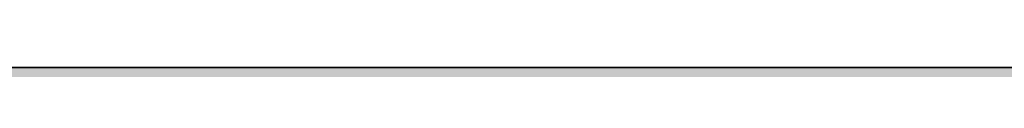
# Model space of a CAD drawing. Units: inches. Extents: x 2091 to 2899, y 967 to 2217.
# Tile 89 of 256: x 2251.29649 to 2251.31428, y 1099.91903 to 1099.91922. Entities that reach past the tile are written whole.
import ezdxf

# ---------------------------------------------------------------- set-up
doc = ezdxf.new("R2010")
doc.units = ezdxf.units.IN
doc.layers.add('A-WALL-PATT', color=141, linetype='Continuous', lineweight=13, true_color=0xadddf7)
doc.layers.add('L-SITE-WALL', color=7, linetype='Continuous', lineweight=35)

msp = doc.modelspace()

# ---------------------------------------------------------------- hatches: boundary and pattern name
at = {"layer": 'A-WALL-PATT'}
h = msp.add_hatch(color=256, dxfattribs=at)
h.dxf.hatch_style = 1
h.paths.add_polyline_path([(2212.143603, 1941.419059), (2387.643603, 1941.419059), (2387.643603, 1824.419059), (2392.143603, 1824.419059), (2392.143603, 1941.419059), (2609.643603, 1941.419059), (2609.643603, 1825.919059), (2614.143603, 1825.919059), (2614.143603, 1941.419059), (2794.143603, 1941.419059), (2794.143603, 1928.762166), (2803.143603, 1928.762166), (2803.143603, 2050.919059), (2203.143603, 2050.919059), (2203.143603, 1900.757859), (2212.143603, 1900.757859)])
h.paths.add_polyline_path([(2212.143603, 1945.919059), (2212.143603, 2041.919059), (2794.143603, 2041.919059), (2794.143603, 1945.919059), (2402.248245, 1945.919059), (2401.102434, 1945.775832), (2398.702434, 1945.775832)], flags=16)
h.paths.add_polyline_path([(2230.229861, 1948.062793), (2227.349861, 1949.502793), (2225.909861, 1951.902793), (2223.989861, 1952.862793), (2223.029861, 1955.262793), (2222.069861, 1959.582793), (2222.069861, 1963.422793), (2223.029861, 1965.662793), (2223.989861, 1965.342793), (2225.58591, 1963.860747), (2226.911533, 1964.957259), (2226.948861, 1965.938793), (2227.778319, 1966.952143), (2228.199916, 1968.878704), (2230.709861, 1964.862793), (2233.589861, 1966.302793), (2233.607309, 1966.331873), (2233.772659, 1964.938205), (2234.633802, 1963.676473), (2235.029861, 1963.902793), (2236.282035, 1965.572358), (2235.989861, 1962.942793), (2237.954512, 1957.540002), (2238.389861, 1957.902793), (2239.215861, 1960.305793), (2238.654565, 1966.38496), (2238.692792, 1966.438069), (2238.840578, 1967.499707), (2238.780291, 1967.687486), (2238.880538, 1967.786763), (2238.666861, 1966.251793), (2239.215861, 1960.305793), (2238.389861, 1957.902793), (2236.949861, 1956.702793), (2234.549861, 1949.982793)], flags=0)
h.paths.add_polyline_path([(2278.011974, 1948.062793), (2276.496427, 1947.873349), (2275.849833, 1947.688608), (2274.651974, 1947.102793)], flags=0)
h.paths.add_polyline_path([(2269.851974, 1955.742793), (2268.276176, 1956.629329), (2270.867302, 1956.348398), (2269.371974, 1958.142793), (2268.714964, 1959.192325), (2270.569833, 1958.728608), (2268.580725, 1961.906087), (2270.811974, 1960.891883), (2270.811974, 1963.422793), (2271.393315, 1964.779256), (2270.291762, 1966.156196), (2271.771974, 1965.662793), (2272.141387, 1966.524757), (2273.929833, 1965.928608), (2275.630385, 1968.054299), (2276.331938, 1966.72186), (2276.520431, 1966.952143), (2276.942029, 1968.878704), (2277.734293, 1967.611082), (2278.139888, 1969.46452), (2279.659124, 1967.033742), (2280.411974, 1966.782793), (2280.949302, 1967.588785), (2281.609833, 1967.368608), (2282.133266, 1968.153758), (2282.349235, 1966.333445), (2282.349849, 1966.332585), (2283.40755, 1968.09542), (2283.712631, 1965.52402), (2284.320221, 1964.633789), (2284.511809, 1964.889239), (2284.234974, 1965.704793), (2284.500472, 1967.318958), (2284.907944, 1965.41742), (2285.396313, 1966.068579), (2285.432833, 1966.290608), (2285.473338, 1966.171279), (2286.353919, 1967.345387), (2286.222007, 1966.158173), (2287.663492, 1968.080154), (2287.713974, 1968.442793), (2288.481599, 1969.016679), (2288.573993, 1968.728897), (2288.917461, 1969.06904), (2288.606833, 1966.837608), (2288.928726, 1963.35131), (2288.934974, 1963.356793), (2288.929731, 1963.340422), (2289.015281, 1962.413869), (2290.111223, 1963.875126), (2290.132833, 1963.942608), (2290.217672, 1964.017058), (2290.111223, 1963.875126), (2289.155833, 1960.891608), (2288.594036, 1959.257227), (2288.571974, 1959.102793), (2289.531974, 1960.542793), (2290.011974, 1962.462793), (2290.19184, 1962.642659), (2289.769833, 1959.688608), (2286.889833, 1957.288608), (2284.489833, 1950.568608), (2283.314658, 1950.046308), (2283.291974, 1949.982793), (2280.290059, 1948.648608), (2281.129833, 1948.648608), (2282.569833, 1948.168608), (2283.204726, 1948.062793), (2278.971974, 1948.062793), (2276.091974, 1949.502793), (2274.651974, 1951.902793), (2272.731974, 1952.862793)], flags=0)
h.paths.add_polyline_path([(2271.158868, 1958.021765), (2272.969833, 1955.848608), (2272.009833, 1960.168608), (2272.009833, 1964.008608), (2272.624426, 1965.442658), (2274.328023, 1963.860747), (2275.653646, 1964.957259), (2275.637743, 1964.53909), (2277.412231, 1966.006888), (2277.032974, 1965.156793), (2276.829924, 1964.975597), (2276.766012, 1963.295014), (2277.449635, 1962.66022), (2279.451974, 1964.862793), (2282.331974, 1966.302793), (2283.529833, 1966.888608), (2283.294512, 1966.770948), (2283.912993, 1963.8847), (2284.899249, 1964.448275), (2284.731974, 1962.942793), (2286.696625, 1957.540002), (2287.131974, 1957.902793), (2287.541913, 1959.095388), (2287.779395, 1958.442311), (2285.682738, 1956.695097), (2285.876503, 1959.795336), (2284.731974, 1962.942793), (2284.899249, 1964.448275), (2283.912993, 1963.8847), (2284.223833, 1962.434116), (2283.424365, 1963.605484), (2281.609833, 1962.568608), (2281.129833, 1960.168608), (2282.089833, 1956.328608), (2283.049833, 1952.968608), (2282.569833, 1950.568608), (2280.169833, 1948.648608), (2279.883316, 1948.791867), (2278.971974, 1948.062793), (2278.971974, 1949.022793), (2278.672313, 1949.397368), (2277.289833, 1950.088608), (2275.849833, 1952.488608), (2273.929833, 1953.448608), (2272.489833, 1954.888608), (2271.921647, 1954.888608), (2271.771974, 1955.262793)], flags=0)
h.paths.add_polyline_path([(2311.994146, 1955.742793), (2312.062717, 1955.674221), (2312.0551, 1955.7085)], flags=0)
h.paths.add_polyline_path([(2331.956146, 1963.951793), (2333.396146, 1965.391793), (2331.077146, 1963.356793), (2330.998603, 1963.111517)], flags=0)
h.paths.add_polyline_path([(2310.554146, 1954.302793), (2307.039807, 1956.279943), (2310.762903, 1955.876284), (2312.474146, 1953.822793), (2313.434146, 1951.422793), (2315.354146, 1950.462793), (2316.794146, 1948.062793), (2317.466146, 1947.726793), (2319.368691, 1947.964611), (2317.754146, 1949.982793), (2317.569531, 1950.610485), (2316.794146, 1951.902793), (2314.874146, 1952.862793), (2313.914146, 1955.262793), (2311.514146, 1958.142793), (2309.375489, 1961.559168), (2311.514146, 1960.337078), (2311.514146, 1961.982793), (2310.604672, 1963.119635), (2311.726605, 1962.47853), (2312.418332, 1964.09256), (2312.255964, 1964.29552), (2313.194146, 1963.982793), (2313.914146, 1965.662793), (2314.646778, 1965.418582), (2315.354146, 1966.302793), (2316.794146, 1967.742793), (2316.157435, 1966.946904), (2317.034111, 1965.28186), (2317.222604, 1965.512143), (2317.777048, 1968.045771), (2318.474111, 1966.72186), (2318.662604, 1966.952143), (2319.084201, 1968.878704), (2321.207049, 1965.482147), (2322.161419, 1966.913702), (2322.554146, 1966.782793), (2322.785988, 1967.130555), (2322.881646, 1966.324293), (2323.312041, 1965.72174), (2323.651289, 1965.891364), (2324.3965, 1967.133382), (2324.656945, 1964.938205), (2324.971986, 1964.476611), (2325.38728, 1967.001499), (2325.940813, 1964.418348), (2327.228929, 1966.135836), (2327.16632, 1965.572358), (2328.059139, 1966.762783), (2328.224576, 1966.247486), (2329.667971, 1967.67691), (2329.664576, 1967.687486), (2329.764823, 1967.786763), (2329.551146, 1966.251793), (2330.100146, 1960.305793), (2329.332814, 1958.07347), (2329.313065, 1957.935225), (2329.634146, 1958.202793), (2330.234146, 1959.102793), (2330.714146, 1961.022793), (2331.034146, 1961.342793), (2330.714146, 1959.102793), (2329.634146, 1958.202793), (2329.274146, 1957.662793), (2327.712112, 1956.361098), (2325.434146, 1949.982793), (2324.333769, 1949.493736), (2323.994146, 1948.542793), (2319.674146, 1946.622793), (2316.794146, 1948.062793), (2315.354146, 1950.462793), (2313.434146, 1951.422793)], flags=0)
h.paths.add_polyline_path([(2321.335684, 1947.952023), (2321.114146, 1948.062793), (2321.114146, 1949.022793), (2319.194146, 1951.422793), (2316.794146, 1959.582793), (2316.663237, 1959.582793), (2315.354146, 1958.142793), (2314.394146, 1958.142793), (2313.148303, 1958.709085), (2312.954146, 1959.582793), (2312.954146, 1960.891883), (2315.834146, 1959.582793), (2316.663237, 1959.582793), (2317.314709, 1960.299412), (2315.030195, 1962.420747), (2316.355818, 1963.517259), (2316.372337, 1963.951615), (2316.470195, 1963.860747), (2317.795818, 1964.957259), (2317.755219, 1963.889687), (2319.175146, 1965.156793), (2319.498407, 1965.881372), (2321.114146, 1965.342793), (2323.235885, 1962.372358), (2325.686349, 1963.772623), (2325.542789, 1962.480576), (2325.198783, 1963.494014), (2324.47851, 1963.082429), (2324.926005, 1960.994116), (2324.078087, 1962.236473), (2322.414791, 1961.286018), (2322.074146, 1959.582793), (2323.034146, 1955.742793), (2323.994146, 1952.382793), (2323.514146, 1949.982793), (2322.142717, 1948.88565), (2322.074146, 1948.542793)], flags=0)
h.paths.add_polyline_path([(2320.207479, 1963.337459), (2320.154146, 1963.422793), (2320.394146, 1963.542793)], flags=0)
h.paths.add_polyline_path([(2353.850527, 1965.8105), (2354.030527, 1965.7505), (2354.330527, 1966.4505), (2354.330527, 1966.9305)], flags=0)
h.paths.add_polyline_path([(2359.020582, 1969.026412), (2359.098382, 1968.901932), (2359.233527, 1969.5195), (2359.233527, 1969.9995)], flags=0)
h.paths.add_polyline_path([(2358.256694, 1966.681672), (2357.983601, 1966.348035), (2358.211267, 1966.146175), (2358.410492, 1966.389568)], flags=0)
h.paths.add_polyline_path([(2357.768473, 1966.058778), (2357.7322, 1965.104967), (2357.751047, 1965.120556), (2357.769527, 1965.6065), (2357.769527, 1966.057843)], flags=0)
h.paths.add_polyline_path([(2359.111527, 1965.3045), (2359.111527, 1964.8245), (2359.844527, 1966.4675), (2359.844527, 1966.9475)], flags=0)
h.paths.add_polyline_path([(2360.223684, 1966.621449), (2360.698527, 1969.3625), (2360.698527, 1969.8425), (2360.210527, 1967.0255), (2360.210527, 1966.6425)], flags=0)
h.paths.add_polyline_path([(2363.450527, 1967.8905), (2363.450527, 1968.3705), (2362.490527, 1966.9305), (2362.656045, 1966.698776)], flags=0)
h.paths.add_polyline_path([(2364.475523, 1966.078826), (2365.850527, 1968.3705), (2365.850527, 1968.8505), (2364.427975, 1966.479581)], flags=0)
h.paths.add_polyline_path([(2366.313527, 1965.8525), (2366.366709, 1965.695829), (2366.802527, 1968.3455), (2366.802527, 1968.8255)], flags=0)
h.paths.add_polyline_path([(2367.16531, 1965.803544), (2367.290527, 1966.9305), (2367.290527, 1967.4105), (2367.102701, 1965.720066)], flags=0)
h.paths.add_polyline_path([(2370.036527, 1959.9735), (2371.013527, 1963.0245), (2371.013527, 1963.5045), (2370.036527, 1960.4535)], flags=0)
h.paths.add_polyline_path([(2371.610527, 1960.2105), (2372.570527, 1961.6505), (2372.570527, 1962.1305), (2371.802527, 1960.9785)], flags=0)
h.paths.add_polyline_path([(2350.873666, 1956.005086), (2351.930527, 1955.8905), (2354.490527, 1953.3305), (2353.850527, 1954.9305), (2351.450527, 1957.8105), (2347.935527, 1963.4255), (2347.935527, 1963.9055), (2351.450527, 1958.2905), (2353.705073, 1955.585046), (2352.890527, 1959.2505), (2352.890527, 1959.7305), (2352.890527, 1961.924786), (2356.730527, 1959.7305), (2358.454471, 1961.626838), (2354.810527, 1965.0105), (2355.030855, 1965.28591), (2358.691091, 1961.88712), (2361.530527, 1965.0105), (2364.376495, 1966.433484), (2364.524394, 1965.186911), (2365.454468, 1963.824181), (2365.881073, 1964.067955), (2365.370527, 1966.4505), (2365.370527, 1966.9305), (2366.810527, 1960.2105), (2366.810527, 1959.7305), (2366.388709, 1952.981409), (2367.770527, 1956.8505), (2368.641225, 1957.576082), (2366.810527, 1962.6105), (2366.810527, 1963.0905), (2368.775179, 1957.68771), (2369.210527, 1958.0505), (2370.001592, 1960.351867), (2369.475232, 1966.052668), (2369.513458, 1966.105777), (2369.514173, 1966.110912), (2369.475232, 1966.532668), (2369.513458, 1966.585777), (2369.614635, 1967.312591), (2369.182527, 1968.6585), (2369.182527, 1969.1385), (2369.600957, 1967.835194), (2369.701204, 1967.934471), (2369.717947, 1968.054743), (2370.145176, 1968.374145), (2369.778707, 1968.011224), (2369.701204, 1967.454471), (2370.468161, 1968.214004), (2369.674936, 1967.265771), (2369.514173, 1966.110912), (2370.036527, 1960.4535), (2370.036527, 1959.9735), (2369.441756, 1958.243191), (2370.650527, 1959.2505), (2371.045821, 1962.017559), (2371.130527, 1962.1305), (2370.650527, 1958.7705), (2367.770527, 1956.3705), (2365.370527, 1949.6505), (2362.079099, 1948.187643), (2363.450527, 1947.7305), (2361.050527, 1947.7305), (2360.090527, 1947.7305), (2357.103861, 1947.357167), (2360.090527, 1948.2105), (2358.170527, 1949.1705), (2356.730527, 1951.5705), (2354.810527, 1952.5305), (2351.930527, 1955.4105)], flags=0)
h.paths.add_polyline_path([(2361.050527, 1948.6905), (2359.130527, 1951.0905), (2356.730527, 1959.2505), (2355.770527, 1959.2505), (2352.890527, 1960.559591), (2352.890527, 1961.444786), (2355.890527, 1959.7305), (2356.730527, 1959.7305), (2356.837194, 1959.367834), (2361.530527, 1964.5305), (2363.248422, 1965.389448), (2364.92531, 1963.041805), (2362.490527, 1961.6505), (2362.063861, 1959.517167), (2362.970527, 1955.8905), (2363.930527, 1952.5305), (2363.930527, 1952.0505), (2363.450527, 1949.6505), (2361.050527, 1947.7305)], flags=0)
h.paths.add_polyline_path([(2359.130527, 1951.5705), (2359.290527, 1951.3705), (2361.050527, 1954.4505), (2361.050527, 1954.9305)], flags=0)
h.paths.add_polyline_path([(2357.219527, 1966.5455), (2356.792527, 1968.8145), (2356.792527, 1969.2945), (2357.219527, 1967.0255)], flags=0)
h.paths.add_polyline_path([(2361.050527, 1954.4505), (2361.530527, 1958.7705), (2361.530527, 1959.2505), (2361.050527, 1954.9305)], flags=0)
h.paths.add_polyline_path([(2402.548287, 1948.486076), (2402.302434, 1948.415832), (2402.590434, 1948.415832)], flags=0)
h.paths.add_polyline_path([(2394.142434, 1956.095832), (2395.685052, 1954.553214), (2396.720495, 1953.970679), (2396.062434, 1955.615832), (2395.241381, 1956.601096), (2395.878904, 1956.441715), (2395.102434, 1959.935832), (2395.102434, 1963.775832), (2396.062434, 1966.015832), (2397.022434, 1965.695832), (2398.618483, 1964.213787), (2399.944106, 1965.310299), (2399.981434, 1966.291832), (2400.810891, 1967.305183), (2401.232489, 1969.231744), (2403.537949, 1965.543008), (2403.941984, 1967.389316), (2404.702434, 1967.135832), (2405.460328, 1966.07478), (2406.622434, 1966.655832), (2406.639882, 1966.684913), (2406.805232, 1965.291245), (2406.925694, 1965.114746), (2407.342434, 1964.975832), (2407.874326, 1965.77367), (2408.1691, 1964.398055), (2409.314608, 1965.925398), (2409.217458, 1965.051054), (2409.445232, 1963.131245), (2410.306374, 1961.869513), (2410.702434, 1962.095832), (2411.442269, 1963.082279), (2411.165434, 1963.897832), (2411.616426, 1966.639757), (2411.725365, 1966.791109), (2411.873151, 1967.852747), (2411.812864, 1968.040526), (2411.913111, 1968.139803), (2411.699434, 1966.604832), (2412.248434, 1960.658832), (2413.225434, 1963.709832), (2414.3779, 1964.72116), (2414.513151, 1965.692747), (2414.452864, 1965.880526), (2414.553111, 1965.979803), (2414.3779, 1964.72116), (2414.519817, 1964.845697), (2414.365365, 1964.631109), (2414.339434, 1964.444832), (2414.888434, 1958.498832), (2414.062434, 1956.095832), (2412.622434, 1954.895832), (2410.17137, 1948.032854), (2410.016719, 1948.084404), (2405.902434, 1946.255832), (2405.902434, 1947.215832), (2405.204252, 1948.08856), (2404.222434, 1948.415832), (2403.262434, 1948.415832), (2400.382434, 1949.855832), (2399.662434, 1951.055832), (2397.982434, 1952.735832), (2397.022434, 1953.215832), (2395.685052, 1954.553214), (2392.656776, 1956.256908)], flags=0)
h.paths.add_polyline_path([(2409.08565, 1964.407441), (2409.130363, 1964.275715), (2409.262434, 1964.495832)], flags=0)
h.paths.add_polyline_path([(2397.742434, 1961.615832), (2398.702434, 1963.855832), (2399.662434, 1963.535832), (2401.426563, 1965.740994), (2401.791415, 1966.5588), (2402.071434, 1965.070832), (2402.835507, 1964.393367), (2403.262398, 1964.9149), (2403.338119, 1964.771086), (2402.615516, 1963.976223), (2402.498612, 1960.902238), (2403.542997, 1959.932452), (2404.413203, 1960.889679), (2404.702434, 1962.335832), (2407.916347, 1964.172354), (2409.520211, 1961.926944), (2410.987085, 1957.893042), (2411.422434, 1958.255832), (2412.047964, 1960.075625), (2412.410341, 1959.079088), (2411.675621, 1958.466821), (2411.662434, 1958.255832), (2411.62607, 1958.425529), (2409.982434, 1957.055832), (2407.582434, 1950.335832), (2403.262434, 1948.415832), (2403.262434, 1949.375832), (2401.342434, 1951.775832), (2399.416508, 1958.323981), (2397.742434, 1959.084923), (2397.742434, 1959.970118), (2397.102434, 1960.335832), (2397.742434, 1960.044923)], flags=0)
h.paths.add_polyline_path([(2405.902434, 1952.975832), (2405.950434, 1953.407832), (2406.016719, 1953.175832)], flags=0)
h.paths.add_polyline_path([(2449.817778, 1967.114014), (2449.752323, 1967.135832), (2449.793703, 1967.077901)], flags=0)
h.paths.add_polyline_path([(2451.697696, 1966.61812), (2451.740895, 1966.690118), (2451.692051, 1966.665696)], flags=0)
h.paths.add_polyline_path([(2454.343628, 1965.737572), (2455.752323, 1967.615832), (2455.992323, 1968.095832), (2454.364497, 1965.925398)], flags=0)
h.paths.add_polyline_path([(2457.547323, 1968.863832), (2457.787323, 1969.343832), (2457.054323, 1968.795832), (2457.007622, 1968.460345)], flags=0)
h.paths.add_polyline_path([(2456.921784, 1967.856662), (2456.802238, 1968.229016), (2456.723, 1967.659803)], flags=0)
h.paths.add_polyline_path([(2457.302323, 1967.376832), (2457.542323, 1967.856832), (2456.810323, 1966.839832), (2456.740516, 1966.700218), (2456.749021, 1966.608105)], flags=0)
h.paths.add_polyline_path([(2458.275323, 1963.709832), (2458.155343, 1963.335153), (2460.354323, 1965.264832), (2460.594323, 1965.744832)], flags=0)
h.paths.add_polyline_path([(2458.392323, 1962.815832), (2458.364088, 1962.618185), (2459.592323, 1964.255832), (2459.832323, 1964.735832)], flags=0)
h.paths.add_polyline_path([(2459.352323, 1962.815832), (2459.272323, 1962.495832), (2460.072323, 1963.295832), (2460.312323, 1963.775832)], flags=0)
h.paths.add_polyline_path([(2458.680323, 1960.607832), (2458.632323, 1960.415832), (2459.592323, 1961.855832), (2459.832323, 1962.335832)], flags=0)
h.paths.add_polyline_path([(2437.83817, 1956.24265), (2439.192323, 1956.095832), (2441.352323, 1953.935832), (2440.872323, 1955.135832), (2438.472323, 1958.015832), (2438.071563, 1958.656023), (2438.712323, 1958.495832), (2440.639596, 1956.183105), (2439.912323, 1959.455832), (2439.912323, 1963.295832), (2441.352323, 1966.655832), (2441.592323, 1967.135832), (2441.112323, 1966.015832), (2442.072323, 1965.695832), (2443.988993, 1968.09167), (2444.241323, 1966.750832), (2444.916801, 1966.15192), (2445.676574, 1967.080136), (2446.255323, 1969.724832), (2446.495323, 1970.204832), (2446.282379, 1969.231744), (2447.362672, 1967.503275), (2447.720323, 1969.567832), (2447.960323, 1970.047832), (2447.48548, 1967.306781), (2448.792323, 1965.215832), (2448.472323, 1964.863832), (2448.552323, 1964.735832), (2451.452051, 1966.185696), (2451.615122, 1964.811245), (2452.307917, 1963.796172), (2453.234505, 1964.325651), (2454.072323, 1960.415832), (2453.628687, 1953.317651), (2454.792323, 1956.575832), (2455.032323, 1957.055832), (2455.718835, 1957.627926), (2453.832323, 1962.815832), (2453.940966, 1963.793615), (2453.335323, 1965.577832), (2453.824323, 1968.550832), (2454.064323, 1969.030832), (2453.575323, 1966.057832), (2454.040333, 1964.687919), (2453.832323, 1962.815832), (2455.718835, 1957.627926), (2456.367207, 1958.168235), (2457.058323, 1960.178832), (2457.298323, 1960.658832), (2456.472323, 1958.255832), (2457.717729, 1959.29367), (2457.672323, 1958.975832), (2454.889951, 1956.657188), (2453.614142, 1953.084923), (2453.592323, 1952.735832), (2453.352323, 1952.255832), (2453.359596, 1952.372196), (2452.632323, 1950.335832), (2452.392323, 1949.855832), (2449.203752, 1948.43869), (2450.712323, 1947.935832), (2448.072323, 1947.935832), (2447.112323, 1947.935832), (2444.552323, 1947.615832), (2447.199596, 1948.372196), (2445.192323, 1949.375832), (2443.752323, 1951.775832), (2441.832323, 1952.735832), (2438.952323, 1955.615832)], flags=0)
h.paths.add_polyline_path([(2443.992323, 1959.935832), (2444.040323, 1959.772632), (2444.121554, 1959.861986)], flags=0)
h.paths.add_polyline_path([(2442.912323, 1959.935832), (2443.032323, 1959.935832), (2442.445657, 1960.202499)], flags=0)
h.paths.add_polyline_path([(2444.982943, 1965.019677), (2445.279323, 1965.264832), (2445.519323, 1965.744832), (2444.993996, 1965.310299)], flags=0)
h.paths.add_polyline_path([(2446.133323, 1965.029832), (2446.330366, 1965.471499), (2444.970323, 1964.257832), (2444.730323, 1963.777832)], flags=0)
h.paths.add_polyline_path([(2442.792323, 1959.455832), (2443.752323, 1959.455832), (2446.152323, 1951.295832), (2446.412323, 1951.750832), (2446.392323, 1951.775832), (2448.080599, 1954.730315), (2448.552323, 1958.975832), (2441.832323, 1965.215832), (2442.154946, 1965.619111), (2448.792323, 1959.455832), (2448.312323, 1955.135832), (2448.072323, 1954.655832), (2446.412323, 1951.750832), (2448.312323, 1949.375832), (2448.312323, 1948.415832), (2450.540895, 1950.19869), (2450.952323, 1952.255832), (2449.992323, 1955.615832), (2449.032323, 1959.455832), (2449.512323, 1961.855832), (2449.752323, 1962.335832), (2449.674904, 1961.948736), (2452.994505, 1963.845651), (2453.064414, 1963.519409), (2452.884611, 1963.782854), (2449.674904, 1961.948736), (2449.272323, 1959.935832), (2450.232323, 1956.095832), (2451.192323, 1952.735832), (2450.712323, 1950.335832), (2450.472323, 1949.855832), (2448.072323, 1947.935832), (2448.072323, 1948.535832), (2445.432323, 1949.855832), (2443.992323, 1952.255832), (2442.072323, 1953.215832), (2441.112323, 1955.615832), (2440.152323, 1959.935832), (2440.152323, 1960.655832)], flags=0)
h.paths.add_polyline_path([(2456.692323, 1966.985832), (2457.608323, 1968.080832), (2457.848323, 1968.560832), (2456.932323, 1967.465832)], flags=0)
h.paths.add_polyline_path([(2489.89657, 1966.580241), (2489.942948, 1966.189347), (2490.747488, 1967.530248), (2491.319122, 1968.951161)], flags=0)
h.paths.add_polyline_path([(2473.562471, 1956.407131), (2477.139981, 1956.019257), (2476.955333, 1956.240834), (2475.108049, 1957.280108), (2476.347488, 1956.970248), (2475.186901, 1958.824216), (2476.919122, 1958.391161), (2475.411642, 1960.799269), (2477.787488, 1959.719339), (2477.787488, 1962.250248), (2477.637399, 1962.43786), (2477.82255, 1962.332059), (2478.359122, 1963.58406), (2478.359122, 1963.671161), (2477.324348, 1964.964628), (2478.714826, 1964.501135), (2479.319122, 1965.911161), (2480.279122, 1965.591161), (2481.783965, 1967.472214), (2482.116488, 1965.705248), (2482.880562, 1965.027782), (2483.209305, 1965.429408), (2483.220169, 1965.71509), (2483.07594, 1965.989022), (2483.711762, 1966.765808), (2484.130488, 1968.679248), (2484.702122, 1970.100161), (2484.489177, 1969.127072), (2486.502904, 1965.905109), (2487.387488, 1965.610248), (2488.153419, 1966.759144), (2488.717017, 1965.970108), (2489.200086, 1966.211642), (2489.330671, 1965.110992), (2490.393905, 1963.622465), (2490.660765, 1963.774956), (2490.493905, 1964.553636), (2490.923063, 1963.924841), (2491.319122, 1964.151161), (2491.333389, 1964.170183), (2491.210488, 1964.532248), (2491.281756, 1964.965537), (2491.425789, 1964.293383), (2494.076476, 1967.827632), (2494.497918, 1966.514942), (2494.598165, 1966.614218), (2494.689488, 1967.270248), (2495.106748, 1967.582196), (2495.129839, 1967.748075), (2495.069552, 1967.935854), (2495.169799, 1968.035131), (2495.031777, 1967.043632), (2495.753818, 1967.758684), (2494.982053, 1966.686437), (2494.956122, 1966.500161), (2495.479021, 1960.836851), (2495.910488, 1962.184248), (2496.482122, 1963.605161), (2496.072694, 1962.326589), (2496.768904, 1962.937536), (2496.599122, 1962.711161), (2496.119122, 1959.351161), (2496.732873, 1960.271787), (2496.987488, 1961.290248), (2497.559122, 1962.711161), (2497.079122, 1960.791161), (2496.507488, 1959.370248), (2495.547488, 1957.930248), (2492.758842, 1955.606376), (2490.839122, 1950.231161), (2490.267488, 1948.810248), (2485.947488, 1946.890248), (2483.067488, 1948.330248), (2481.627488, 1950.730248), (2479.707488, 1951.690248), (2476.827488, 1954.570248)], flags=0)
h.paths.add_polyline_path([(2485.576973, 1948.313392), (2485.559122, 1948.311161), (2485.578758, 1948.311161)], flags=0)
h.paths.add_polyline_path([(2478.645063, 1954.551161), (2478.109042, 1956.963257), (2479.319122, 1955.511161), (2480.279122, 1953.111161), (2482.199122, 1952.151161), (2483.639122, 1949.751161), (2486.519122, 1948.311161), (2486.519122, 1949.271161), (2484.739307, 1951.49593), (2484.027488, 1950.250248), (2481.627488, 1958.410248), (2482.375148, 1959.232673), (2482.199122, 1959.831161), (2483.197572, 1960.929456), (2479.707488, 1964.170248), (2480.603358, 1965.290085), (2481.875171, 1964.109115), (2482.666387, 1964.763582), (2482.615359, 1963.421798), (2482.989199, 1963.074661), (2484.008488, 1963.984248), (2484.683606, 1965.497507), (2484.580122, 1965.405161), (2485.357268, 1967.147113), (2485.120645, 1965.781197), (2486.427488, 1963.690248), (2488.145383, 1964.549195), (2489.822271, 1962.201552), (2490.747488, 1962.730248), (2491.999662, 1964.399813), (2492.076046, 1965.087265), (2492.212892, 1964.684119), (2492.485374, 1965.047429), (2492.279122, 1963.191161), (2494.243773, 1957.78837), (2494.562503, 1958.053978), (2494.933488, 1959.133248), (2495.505122, 1960.554161), (2494.679122, 1958.151161), (2494.107488, 1956.730248), (2494.562503, 1958.053978), (2493.408544, 1957.092345), (2491.707488, 1961.770248), (2491.999662, 1964.399813), (2490.747488, 1962.730248), (2487.71203, 1960.9957), (2487.479122, 1959.831161), (2488.439122, 1955.991161), (2489.399122, 1952.631161), (2488.919122, 1950.231161), (2488.576918, 1949.957397), (2488.347488, 1948.810248), (2487.651715, 1948.253629), (2487.479122, 1948.311161), (2486.519122, 1948.311161), (2483.639122, 1949.751161), (2482.199122, 1952.151161), (2480.279122, 1953.111161), (2478.839122, 1954.551161)], flags=0)
h.paths.add_polyline_path([(2526.648252, 1966.987524), (2526.517343, 1967.031161), (2526.600102, 1966.915298)], flags=0)
h.paths.add_polyline_path([(2528.47064, 1966.446656), (2528.574486, 1966.619732), (2528.457071, 1966.561025)], flags=0)
h.paths.add_polyline_path([(2534.133343, 1967.496161), (2534.156685, 1967.542845), (2534.059841, 1967.408296)], flags=0)
h.paths.add_polyline_path([(2536.161923, 1964.0506), (2535.157343, 1962.711161), (2535.100872, 1962.315866), (2536.117343, 1963.671161), (2536.420532, 1964.277539)], flags=0)
h.paths.add_polyline_path([(2535.157343, 1959.831161), (2536.117343, 1961.271161), (2536.597343, 1962.231161), (2535.253343, 1960.215161)], flags=0)
h.paths.add_polyline_path([(2513.249035, 1956.284796), (2516.221181, 1955.962555), (2514.997343, 1957.431161), (2514.195823, 1958.711541), (2515.477343, 1958.391161), (2516.931888, 1956.645706), (2516.437343, 1958.871161), (2516.437343, 1962.711161), (2516.872692, 1963.726974), (2515.346434, 1965.634797), (2517.397343, 1964.951161), (2517.877343, 1966.071161), (2518.357343, 1967.031161), (2517.877343, 1965.911161), (2518.837343, 1965.591161), (2520.48659, 1967.652719), (2520.766343, 1966.166161), (2521.530417, 1965.488695), (2521.781443, 1965.795375), (2521.800911, 1966.307268), (2521.477804, 1966.920936), (2521.246343, 1967.126161), (2521.177701, 1967.490913), (2521.477804, 1966.920936), (2522.010417, 1966.448695), (2522.257386, 1966.750417), (2522.780343, 1969.140161), (2523.260343, 1970.100161), (2523.047398, 1969.127072), (2524.673132, 1966.525897), (2526.037343, 1966.071161), (2526.795238, 1965.010108), (2527.977071, 1965.601025), (2528.140141, 1964.226573), (2528.66459, 1963.458159), (2529.388616, 1963.871888), (2529.329665, 1964.14699), (2529.481284, 1963.924841), (2529.877343, 1964.151161), (2529.98401, 1964.293383), (2529.789053, 1965.20318), (2530.0624, 1964.397903), (2532.802483, 1968.051347), (2533.147773, 1966.975854), (2533.24802, 1967.075131), (2533.339343, 1967.731161), (2533.672848, 1967.980493), (2533.72802, 1968.035131), (2533.514343, 1966.500161), (2534.024718, 1960.972496), (2534.560343, 1962.645161), (2535.040343, 1963.605161), (2534.063343, 1960.554161), (2533.237343, 1958.151161), (2534.288154, 1959.026836), (2534.197343, 1958.391161), (2531.512597, 1956.153872), (2529.397343, 1950.231161), (2528.917343, 1949.271161), (2526.448772, 1948.174018), (2527.477343, 1947.831161), (2530.357343, 1947.351161), (2524.597343, 1947.351161), (2521.717343, 1948.791161), (2520.277343, 1951.191161), (2518.357343, 1952.151161), (2515.477343, 1955.031161)], flags=0)
h.paths.add_polyline_path([(2523.93476, 1967.190308), (2523.619512, 1966.483689), (2523.7705, 1966.242109)], flags=0)
h.paths.add_polyline_path([(2518.837343, 1953.111161), (2517.877343, 1955.511161), (2516.884983, 1959.976779), (2516.917343, 1959.96207), (2516.917343, 1962.025446), (2520.757343, 1959.831161), (2522.024949, 1961.225527), (2518.357343, 1964.631161), (2519.002589, 1965.437718), (2520.433392, 1964.109115), (2521.30112, 1964.826871), (2521.245157, 1963.355333), (2525.638307, 1959.27598), (2526.037343, 1961.271161), (2529.397343, 1963.191161), (2530.649517, 1964.860726), (2530.66472, 1964.99755), (2530.691956, 1964.917311), (2531.087778, 1965.445074), (2530.945985, 1964.168944), (2530.691956, 1964.917311), (2529.397343, 1963.191161), (2526.362504, 1961.456967), (2526.037343, 1959.831161), (2526.997343, 1955.991161), (2527.957343, 1952.631161), (2527.477343, 1950.231161), (2527.134486, 1949.956875), (2526.973928, 1949.154087), (2526.697343, 1949.031161), (2524.597343, 1947.351161), (2524.597343, 1948.311161), (2524.277343, 1948.711161), (2522.197343, 1949.751161), (2520.757343, 1952.151161)], flags=0)
h.paths.add_polyline_path([(2520.277343, 1958.871161), (2520.853343, 1959.504761), (2523.157343, 1951.671161), (2524.613895, 1954.220126), (2524.597343, 1954.071161), (2522.677343, 1950.711161)], flags=0)
h.paths.add_polyline_path([(2559.37091, 1966.311161), (2559.398411, 1966.324911), (2559.401943, 1966.345296)], flags=0)
h.paths.add_polyline_path([(2549.77091, 1957.191161), (2552.65091, 1954.311161), (2552.133987, 1955.603468), (2550.61091, 1957.431161), (2547.09591, 1963.046161), (2545.77591, 1965.206161), (2549.29091, 1959.591161), (2551.69091, 1956.711161), (2550.792933, 1960.752059), (2550.73091, 1960.780251), (2550.73091, 1964.871161), (2551.69091, 1967.111161), (2552.65091, 1966.791161), (2554.246959, 1965.309115), (2555.034252, 1965.960337), (2555.581671, 1966.644612), (2555.60991, 1967.387161), (2556.439368, 1968.400511), (2556.860966, 1970.327072), (2559.37091, 1966.311161), (2560.69091, 1964.151161), (2562.408805, 1965.010108), (2561.65091, 1966.071161), (2560.33091, 1968.231161), (2561.758497, 1966.23254), (2562.347213, 1967.115614), (2562.433709, 1966.386573), (2563.127798, 1965.369604), (2563.57091, 1965.591161), (2563.588359, 1965.620241), (2563.362543, 1967.52354), (2563.722489, 1965.843792), (2565.060001, 1968.072979), (2564.732862, 1965.128722), (2565.117577, 1963.333383), (2567.444622, 1966.436109), (2567.315615, 1967.833328), (2567.353841, 1967.886437), (2567.501627, 1968.948075), (2567.44134, 1969.135854), (2567.541587, 1969.235131), (2567.32791, 1967.700161), (2567.87691, 1961.754161), (2568.746689, 1964.470327), (2568.635615, 1965.673328), (2568.673841, 1965.726437), (2568.821627, 1966.788075), (2568.76134, 1966.975854), (2568.861587, 1967.075131), (2568.64791, 1965.540161), (2568.726127, 1964.693026), (2568.85391, 1964.805161), (2568.746689, 1964.470327), (2568.817236, 1963.706261), (2568.97091, 1963.911161), (2568.866075, 1963.17731), (2569.19691, 1959.594161), (2568.37091, 1957.191161), (2566.93091, 1955.991161), (2564.620272, 1949.521373), (2564.65091, 1949.511161), (2564.616625, 1949.511161), (2564.53091, 1949.271161), (2560.21091, 1947.351161), (2557.33091, 1948.791161), (2556.045196, 1950.934018), (2556.01091, 1950.951161), (2555.856625, 1951.208303), (2553.97091, 1952.151161), (2551.09091, 1955.031161), (2546.650144, 1957.529515)], flags=0)
h.paths.add_polyline_path([(2567.025794, 1959.33023), (2567.035007, 1959.304895), (2567.05091, 1959.351161)], flags=0)
h.paths.add_polyline_path([(2551.968287, 1962.518374), (2553.01091, 1964.951161), (2553.97091, 1964.631161), (2555.566959, 1963.149115), (2556.892583, 1964.245627), (2556.92991, 1965.227161), (2557.143984, 1965.488695), (2556.420066, 1966.130557), (2556.391421, 1966.104995), (2556.37991, 1966.166161), (2556.420066, 1966.130557), (2556.95191, 1966.605161), (2557.092139, 1966.919478), (2557.570875, 1966.010228), (2557.759368, 1966.240511), (2557.41791, 1964.680161), (2556.892583, 1964.245627), (2556.807089, 1961.997566), (2560.69091, 1958.391161), (2560.635526, 1957.892699), (2560.81091, 1957.191161), (2561.77091, 1953.831161), (2561.29091, 1951.431161), (2559.110423, 1949.68677), (2559.156484, 1949.629193), (2563.02652, 1951.349209), (2562.61091, 1949.271161), (2560.21091, 1947.351161), (2560.21091, 1948.311161), (2559.25091, 1949.511161), (2558.89091, 1949.511161), (2558.89091, 1949.961161), (2558.29091, 1950.711161), (2558.053701, 1951.517672), (2556.97091, 1952.871161), (2555.06788, 1959.341464), (2552.05091, 1961.065446), (2552.05091, 1962.471161)], flags=0)
h.paths.add_polyline_path([(2588.330049, 1958.391161), (2588.610248, 1958.110962), (2588.553362, 1958.366949)], flags=0)
h.paths.add_polyline_path([(2594.745454, 1950.493086), (2593.957532, 1953.172022), (2593.130049, 1954.551161), (2591.210049, 1955.511161), (2590.250049, 1957.911161), (2588.309033, 1960.240379), (2586.177306, 1961.209346), (2587.850049, 1960.791161), (2587.253416, 1961.744246), (2588.441314, 1961.065446), (2588.441314, 1962.655528), (2588.421679, 1962.665345), (2588.441314, 1962.711161), (2586.914038, 1964.620256), (2588.877086, 1963.727962), (2589.290049, 1964.69154), (2589.290049, 1966.071161), (2590.250049, 1968.311161), (2591.210049, 1967.991161), (2592.806098, 1966.509115), (2594.131721, 1967.605627), (2594.169049, 1968.587161), (2594.998506, 1969.600511), (2595.420104, 1971.527072), (2597.930049, 1967.511161), (2600.810049, 1968.951161), (2600.827497, 1968.980241), (2600.992847, 1967.586573), (2601.853989, 1966.324841), (2602.107143, 1966.4695), (2602.236354, 1967.255069), (2602.356715, 1966.693383), (2603.502223, 1968.220726), (2603.210049, 1965.591161), (2605.1747, 1960.18837), (2605.506891, 1960.465196), (2605.026019, 1965.673328), (2605.064245, 1965.726437), (2605.212031, 1966.788075), (2605.151744, 1966.975854), (2605.251991, 1967.075131), (2605.343314, 1967.731161), (2605.952905, 1968.186898), (2605.874753, 1969.033328), (2605.912979, 1969.086437), (2606.060766, 1970.148075), (2606.000479, 1970.335854), (2606.100725, 1970.435131), (2605.887049, 1968.900161), (2606.436049, 1962.954161), (2605.610049, 1960.551161), (2605.997036, 1960.87365), (2606.564314, 1962.645161), (2608.241494, 1964.116941), (2608.010049, 1963.191161), (2607.050049, 1961.751161), (2606.631486, 1961.402358), (2606.201314, 1958.391161), (2603.321314, 1955.991161), (2600.921314, 1949.271161), (2596.601314, 1947.351161), (2593.721314, 1948.791161), (2592.857314, 1950.231161), (2592.650049, 1950.231161)], flags=0)
h.paths.add_polyline_path([(2596.601314, 1947.351161), (2596.601314, 1948.311161), (2594.681314, 1950.711161), (2596.154954, 1953.290029), (2595.530049, 1954.071161), (2593.199226, 1961.995957), (2592.65134, 1962.504708), (2591.780151, 1963.002531), (2593.282987, 1964.245627), (2593.320314, 1965.227161), (2594.149772, 1966.240511), (2594.57137, 1968.167072), (2596.182651, 1965.589023), (2596.951273, 1966.434508), (2598.041314, 1966.071161), (2598.799209, 1965.010108), (2599.961314, 1965.591161), (2599.978763, 1965.620241), (2600.144113, 1964.226573), (2601.005255, 1962.964841), (2601.401314, 1963.191161), (2602.653488, 1964.860726), (2602.361314, 1962.231161), (2603.792748, 1958.294719), (2601.977644, 1953.212427), (2601.946208, 1952.709453), (2599.468755, 1951.608363), (2599.001314, 1949.271161)], flags=0)
h.paths.add_polyline_path([(2597.561314, 1958.871161), (2597.670966, 1959.419419), (2597.595054, 1958.736204)], flags=0)
h.paths.add_polyline_path([(2623.666305, 1961.254375), (2625.519163, 1960.791161), (2624.965544, 1961.675533), (2627.199163, 1960.660251), (2627.199163, 1961.151161), (2626.959163, 1962.231161), (2626.959163, 1963.491161), (2625.582321, 1965.212213), (2626.959163, 1964.425446), (2626.959163, 1965.831161), (2626.869163, 1965.861161), (2627.919163, 1968.311161), (2628.879163, 1967.991161), (2630.475212, 1966.509115), (2631.800835, 1967.605627), (2631.838163, 1968.587161), (2632.667621, 1969.600511), (2633.089218, 1971.527072), (2635.599163, 1967.511161), (2638.479163, 1968.951161), (2638.496611, 1968.980241), (2638.661961, 1967.586573), (2639.176273, 1966.833011), (2639.780216, 1967.839582), (2640.02583, 1966.693383), (2641.171337, 1968.220726), (2640.879163, 1965.591161), (2641.114265, 1964.94463), (2641.411337, 1965.340726), (2641.308099, 1964.411586), (2642.843814, 1960.18837), (2643.279163, 1960.551161), (2644.084736, 1962.894736), (2643.783867, 1966.153328), (2643.806834, 1966.185237), (2643.600676, 1968.418053), (2643.522812, 1968.660581), (2643.72988, 1970.148075), (2643.669593, 1970.335854), (2643.76984, 1970.435131), (2643.556163, 1968.900161), (2643.600676, 1968.418053), (2643.909593, 1967.455854), (2644.00984, 1967.555131), (2643.811743, 1966.132079), (2644.105163, 1962.954161), (2644.238773, 1961.350836), (2644.719163, 1961.751161), (2645.032853, 1962.221695), (2645.322163, 1963.125161), (2646.07642, 1963.787047), (2645.032853, 1962.221695), (2644.345163, 1960.074161), (2643.519163, 1957.671161), (2642.079163, 1956.471161), (2639.719612, 1949.864419), (2639.875527, 1949.838433), (2635.359163, 1947.831161), (2632.479163, 1949.271161), (2631.039163, 1951.671161), (2629.119163, 1952.631161), (2628.159163, 1955.031161), (2625.759163, 1957.911161)], flags=0)
h.paths.add_polyline_path([(2627.816306, 1956.574018), (2627.373708, 1958.565706), (2626.376306, 1959.762589), (2627.199163, 1959.351161), (2627.373708, 1958.565706), (2627.919163, 1957.911161), (2628.879163, 1955.511161), (2630.799163, 1954.551161), (2632.239163, 1952.151161), (2633.315025, 1951.613229), (2631.039163, 1959.351161), (2631.49783, 1959.855694), (2630.799163, 1962.231161), (2631.449867, 1962.946935), (2630.715212, 1963.629115), (2632.040835, 1964.725627), (2632.078163, 1965.707161), (2632.292237, 1965.968695), (2631.705339, 1966.489067), (2633.136441, 1967.766144), (2633.329218, 1968.647072), (2634.674718, 1966.494272), (2635.208465, 1967.081393), (2636.799163, 1966.551161), (2637.676404, 1967.867023), (2638.993946, 1966.022465), (2639.705345, 1966.428979), (2641.119163, 1959.831161), (2640.930072, 1956.805706), (2639.439163, 1952.631161), (2638.227456, 1952.092624), (2637.759163, 1949.751161), (2635.359163, 1947.831161), (2635.359163, 1948.791161), (2633.439163, 1951.191161), (2633.315025, 1951.613229), (2632.239163, 1952.151161), (2630.799163, 1954.551161), (2628.879163, 1955.511161)], flags=0)
h.paths.add_polyline_path([(2637.759163, 1953.831161), (2637.279163, 1955.511161), (2636.319163, 1959.351161), (2636.799163, 1961.751161), (2639.233946, 1963.142465), (2637.557058, 1965.490108), (2638.738891, 1966.081025), (2638.901961, 1964.706573), (2639.763104, 1963.444841), (2636.799163, 1961.751161), (2636.532496, 1960.417827), (2637.039163, 1958.391161), (2637.999163, 1955.031161)], flags=0)
h.paths.add_polyline_path([(2668.567407, 1951.431161), (2667.607407, 1953.831161), (2665.207407, 1956.711161), (2662.293903, 1961.365307), (2665.447407, 1959.591161), (2666.647407, 1958.391161), (2666.647407, 1959.975161), (2666.058317, 1960.68207), (2666.647407, 1960.345446), (2666.647407, 1961.991161), (2666.70009, 1962.114087), (2666.407407, 1963.431161), (2666.407407, 1967.271161), (2667.367407, 1969.511161), (2668.327407, 1969.191161), (2669.923457, 1967.709115), (2671.24908, 1968.805627), (2671.286407, 1969.787161), (2672.115865, 1970.800511), (2672.537463, 1972.727072), (2675.047407, 1968.711161), (2677.927407, 1970.151161), (2677.944856, 1970.180241), (2678.110206, 1968.786573), (2678.971348, 1967.524841), (2679.367407, 1967.751161), (2680.619581, 1969.420726), (2680.327407, 1966.791161), (2682.292059, 1961.38837), (2682.727407, 1961.751161), (2683.358306, 1963.586571), (2683.232112, 1964.953328), (2683.270338, 1965.006437), (2683.393215, 1965.889138), (2683.359969, 1966.249215), (2683.357837, 1966.255854), (2683.359229, 1966.257232), (2682.992112, 1970.233328), (2683.030338, 1970.286437), (2683.178124, 1971.348075), (2683.117837, 1971.535854), (2683.218084, 1971.635131), (2683.004407, 1970.100161), (2683.359229, 1966.257232), (2683.458084, 1966.355131), (2683.393215, 1965.889138), (2683.413908, 1965.665023), (2684.42381, 1966.872275), (2683.553407, 1964.154161), (2683.358306, 1963.586571), (2683.793407, 1958.874161), (2682.967407, 1956.471161), (2681.527407, 1955.271161), (2680.109226, 1951.300251), (2680.084933, 1950.911573), (2679.976846, 1950.929587), (2679.127407, 1948.551161), (2674.807407, 1946.631161), (2671.927407, 1948.071161), (2670.487407, 1950.471161)], flags=0)
h.paths.add_polyline_path([(2671.935683, 1953.227023), (2671.687407, 1953.351161), (2670.247407, 1955.751161), (2668.327407, 1956.711161), (2667.356741, 1959.137827), (2669.527407, 1958.151161), (2670.487407, 1958.151161), (2671.479407, 1959.242361), (2670.684402, 1961.94538), (2668.889599, 1963.611982), (2667.307407, 1964.331161), (2668.567407, 1963.911161), (2668.830937, 1964.240572), (2670.247407, 1963.431161), (2672.42214, 1965.823367), (2672.777463, 1967.447072), (2673.234074, 1966.716494), (2674.411919, 1968.012124), (2673.980564, 1965.522109), (2675.287407, 1963.431161), (2675.554074, 1963.564494), (2675.932407, 1965.456161), (2676.247407, 1965.351161), (2677.005302, 1964.290108), (2678.167407, 1964.871161), (2679.607407, 1967.271161), (2680.327407, 1963.911161), (2680.306552, 1963.57748), (2680.347242, 1963.457607), (2680.859581, 1964.140726), (2680.567407, 1961.511161), (2681.103624, 1960.036566), (2678.887407, 1953.831161), (2677.092478, 1953.033414), (2677.687407, 1950.951161), (2677.207407, 1948.551161), (2674.807407, 1946.631161), (2674.807407, 1947.591161), (2672.887407, 1949.991161)], flags=0)
h.paths.add_polyline_path([(2673.98455, 1951.911161), (2674.567407, 1952.931161), (2674.567407, 1951.911161), (2676.967407, 1953.831161), (2677.447407, 1956.231161), (2676.487407, 1959.591161), (2676.247407, 1960.551161), (2679.729589, 1962.540979), (2680.059267, 1961.002484), (2679.211348, 1962.244841), (2676.247407, 1960.551161), (2676.487407, 1959.591161), (2677.447407, 1956.231161), (2676.967407, 1953.831161), (2674.567407, 1951.911161)], flags=0)
h.paths.add_polyline_path([(2707.479283, 1952.814651), (2706.519283, 1955.214651), (2705.559283, 1959.534651), (2705.559283, 1963.374651), (2706.519283, 1965.614651), (2707.479283, 1965.294651), (2709.075332, 1963.812605), (2710.400956, 1964.909117), (2710.438283, 1965.890651), (2711.267741, 1966.904001), (2711.689338, 1968.830563), (2714.199283, 1964.814651), (2717.079283, 1966.254651), (2717.096731, 1966.283731), (2717.262082, 1964.890063), (2718.123224, 1963.628331), (2718.519283, 1963.854651), (2719.771457, 1965.524216), (2719.479283, 1962.894651), (2721.443934, 1957.49186), (2721.879283, 1957.854651), (2722.705283, 1960.257651), (2722.143988, 1966.336818), (2722.182214, 1966.389928), (2722.33, 1967.451565), (2722.269713, 1967.639345), (2722.36996, 1967.738621), (2722.156283, 1966.203651), (2722.705283, 1960.257651), (2721.879283, 1957.854651), (2720.439283, 1956.654651), (2718.039283, 1949.934651), (2713.719283, 1948.014651), (2710.839283, 1949.454651), (2709.399283, 1951.854651)], flags=0)
h.paths.add_polyline_path([(2749.301231, 1952.814651), (2748.341231, 1955.214651), (2747.381231, 1959.534651), (2747.381231, 1963.374651), (2748.341231, 1965.614651), (2749.301231, 1965.294651), (2750.89728, 1963.812605), (2752.222903, 1964.909117), (2752.260231, 1965.890651), (2753.089688, 1966.904001), (2753.511286, 1968.830563), (2756.021231, 1964.814651), (2758.901231, 1966.254651), (2758.918679, 1966.283731), (2759.084029, 1964.890063), (2759.945171, 1963.628331), (2760.341231, 1963.854651), (2761.593405, 1965.524216), (2761.301231, 1962.894651), (2763.265882, 1957.49186), (2763.701231, 1957.854651), (2764.527231, 1960.257651), (2763.965935, 1966.336818), (2764.004161, 1966.389928), (2764.151948, 1967.451565), (2764.091661, 1967.639345), (2764.191907, 1967.738621), (2763.978231, 1966.203651), (2764.527231, 1960.257651), (2763.701231, 1957.854651), (2762.261231, 1956.654651), (2759.861231, 1949.934651), (2755.541231, 1948.014651), (2752.661231, 1949.454651), (2751.221231, 1951.854651)], flags=0)
h.paths.add_polyline_path([(2212.143603, 1819.934514), (2203.143603, 1819.934514), (2203.143603, 1739.979546), (2212.143603, 1739.979546), (2212.143603, 1780.919059), (2392.143603, 1780.919059), (2392.143603, 1783.919059), (2212.143603, 1783.919059)])
h.paths.add_polyline_path([(2803.143603, 1847.938821), (2794.143603, 1847.938821), (2794.143603, 1785.419059), (2609.643603, 1785.419059), (2493.875609, 1785.419059), (2493.875609, 1780.919059), (2609.643603, 1780.919059), (2794.143603, 1780.919059), (2794.143603, 1696.919059), (2609.375609, 1696.919059), (2609.375609, 1742.919059), (2604.875609, 1742.919059), (2604.875609, 1644.419059), (2609.375609, 1644.419059), (2609.375609, 1692.419059), (2794.143603, 1692.419059), (2794.143603, 1668.164737), (2803.143603, 1668.164737)])
h.paths.add_polyline_path([(2392.143603, 1740.419059), (2387.643603, 1740.419059), (2387.643603, 1629.419059), (2212.143603, 1629.419059), (2212.143603, 1659.156202), (2203.143603, 1659.156202), (2203.143603, 1494.089439), (2212.143603, 1494.089439), (2212.143603, 1627.919059), (2392.143603, 1627.919059)])
h.paths.add_polyline_path([(2457.875609, 1780.919059), (2453.375609, 1780.919059), (2453.375609, 1644.419059), (2568.875609, 1644.419059), (2568.875609, 1648.919059), (2457.875609, 1648.919059)])
h.paths.add_polyline_path([(2545.143603, 1591.919059), (2540.643603, 1591.919059), (2540.643603, 1567.919059), (2468.643603, 1567.919059), (2468.643603, 1627.919059), (2509.143603, 1627.919059), (2509.143603, 1632.419059), (2464.143603, 1632.419059), (2464.143603, 1563.419059), (2545.143603, 1563.419059)])
h.paths.add_polyline_path([(2268.643603, 1555.919059), (2212.143603, 1555.919059), (2212.143603, 1551.419059), (2268.643603, 1551.419059)], flags=17)
h.paths.add_polyline_path([(2212.143603, 1413.266094), (2203.143603, 1413.266094), (2203.143603, 1233.070405), (2212.143603, 1233.070405)])
h.paths.add_polyline_path([(2267.643603, 1351.919059), (2212.143603, 1351.919059), (2212.143603, 1347.419059), (2267.643603, 1347.419059)], flags=17)
h.paths.add_polyline_path([(2456.643603, 1489.419059), (2452.143603, 1489.419059), (2452.143603, 1351.919059), (2312.643603, 1351.919059), (2312.643603, 1347.419059), (2456.643603, 1347.419059)])
h.paths.add_polyline_path([(2472.370171, 1455.419059), (2467.870171, 1455.419059), (2467.870171, 1347.419059), (2472.370171, 1347.419059)])
h.paths.add_polyline_path([(2794.143603, 1351.919059), (2543.370171, 1351.919059), (2543.370171, 1347.419059), (2794.143603, 1347.419059)], flags=17)
h.paths.add_polyline_path([(2312.643603, 1347.419059), (2308.143603, 1347.419059), (2308.143603, 1302.161787), (2308.341966, 1302.164327), (2308.143603, 1298.169249), (2308.143603, 1275.419059), (2212.143603, 1275.419059), (2212.143603, 1270.919059), (2312.643603, 1270.919059)], flags=17)
h.paths.add_polyline_path([(2212.143603, 1152.24706), (2203.143603, 1152.24706), (2203.143603, 1090.919059), (2803.143603, 1090.919059), (2803.143603, 1392.713555), (2794.143603, 1392.713555), (2794.143603, 1143.419059), (2548.032447, 1143.419059), (2548.032447, 1138.919059), (2794.143603, 1138.919059), (2794.143603, 1099.919059), (2212.143603, 1099.919059)])
h.paths.add_polyline_path([(2471.532447, 1266.328529, 0.031658), (2467.032447, 1269.945786), (2467.032447, 1143.419059), (2471.532447, 1143.419059), (2471.532447, 1148.819059)], flags=17)
h.paths.add_polyline_path([(2803.143603, 1587.341392), (2794.143603, 1587.341392), (2794.143603, 1473.5369), (2803.143603, 1473.5369)])
h.paths.add_polyline_path([(2794.143603, 1536.419059), (2651.143603, 1536.419059), (2651.143603, 1531.919059), (2794.143603, 1531.919059)])
h.paths.add_polyline_path([(2614.143603, 1620.419059), (2609.643603, 1620.419059), (2609.643603, 1536.419059), (2614.143603, 1536.419059)])
h.paths.add_polyline_path([(2271.082728, 1964.317238), (2776.852968, 1964.317238), (2776.852968, 2037.169623), (2271.082728, 2037.169623)], flags=8)
h.paths.add_polyline_path([(2380.649285, 1536.824144), (2461.040809, 1536.824144), (2461.040809, 1554.652587), (2380.649285, 1554.652587)], flags=9)
h.paths.add_polyline_path([(2203.655038, 1608.815312), (2316.118439, 1608.815312), (2316.118439, 1621.918356), (2203.655038, 1621.918356)], flags=24)
h.paths.add_polyline_path([(2212.677255, 1313.504102), (2282.59152, 1313.504102), (2282.59152, 1322.745239), (2212.677255, 1322.745239)], flags=24)
h.paths.add_polyline_path([(2457.111976, 1114.778574), (2558.481581, 1114.778574), (2558.481581, 1142.219682), (2457.111976, 1142.219682)], flags=25)
h.paths.add_polyline_path([(2473.442337, 1273.010067), (2604.641226, 1273.010067), (2604.641226, 1318.346935), (2473.442337, 1318.346935)], flags=25)
h.paths.add_polyline_path([(2638.876302, 1626.977432), (2684.250367, 1627.976738), (2684.038483, 1637.597494), (2638.664417, 1636.598188)], flags=9)
h.paths.add_polyline_path([(2537.590554, 1453.793447), (2628.389547, 1453.793447), (2628.389547, 1475.344811), (2537.590554, 1475.344811)], flags=9)
h.paths.add_polyline_path([(2504.137638, 1714.632397), (2554.647187, 1714.632397), (2554.647187, 1730.237712), (2504.137638, 1730.237712)], flags=25)
h.paths.add_polyline_path([(2487.501181, 1575.651872), (2535.097121, 1575.651872), (2535.097121, 1598.377646), (2487.501181, 1598.377646)], flags=25)
h.paths.add_polyline_path([(2709.0994, 1735.710278), (2740.016601, 1735.710278), (2740.016601, 1749.937641), (2709.0994, 1749.937641)], flags=25)
h.paths.add_polyline_path([(2442.438424, 1792.171657), (2564.728835, 1792.171657), (2564.728835, 1842.000163), (2442.438424, 1842.000163)], flags=9)
h.paths.add_polyline_path([(2655.815801, 1809.644076), (2789.520142, 1806.693796), (2790.084977, 1832.291638), (2656.380635, 1835.241918)], flags=25)
h.paths.add_polyline_path([(2234.842697, 1797.720143), (2368.592851, 1794.768852), (2369.160718, 1820.504132), (2235.410564, 1823.455423)], flags=9)
h.paths.add_polyline_path([(2245.138466, 1644.006335), (2398.427733, 1640.6239), (2398.994842, 1666.32482), (2245.705575, 1669.707255)], flags=9)
h.paths.add_polyline_path([(2306.142847, 1431.168519), (2413.768314, 1428.793687), (2414.333148, 1454.391529), (2306.707682, 1456.76636)], flags=9)
h.paths.add_polyline_path([(2306.834582, 1458.233145), (2393.380484, 1456.323449), (2393.932808, 1481.354358), (2307.386907, 1483.264054)], flags=9)

# ---------------------------------------------------------------- linework, layer by layer
at = {"layer": 'L-SITE-WALL'}
msp.add_line((2794.143603, 1099.919059), (2212.143603, 1099.919059), dxfattribs=at)

doc.saveas('drawing.dxf')
